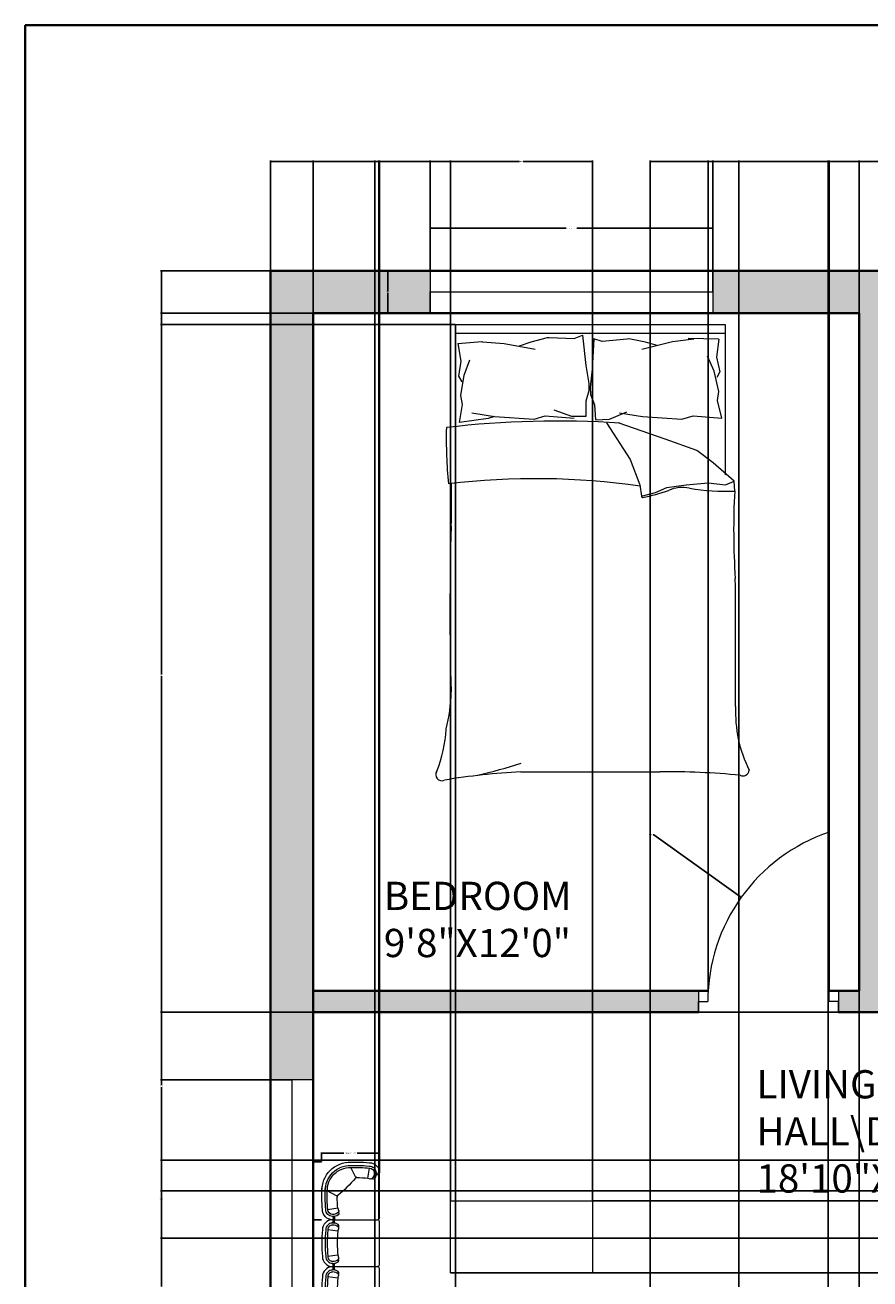
# Model space of a CAD drawing. Units: inches. Extents: x 2606 to 3027, y 1906 to 2463.
# Tile 5 of 10: x 2606 to 2785, y 2196 to 2463. Entities that reach past the tile are written whole.
import ezdxf

# ---------------------------------------------------------------- set-up
doc = ezdxf.new("R2010")
doc.units = ezdxf.units.IN
for name, color, linetype, lineweight in [('A-ANNO-DIMS', 2, 'Continuous', 18), ('A-ANNO-TTLB', 7, 'Continuous', 35), ('A-AREA-IDEN', 7, 'Continuous', 18), ('A-DOOR', 3, 'Continuous', 18), ('A-FURN', 8, 'Continuous', 13), ('A-GLAZ', 4, 'Continuous', 18), ('A-WALL', 7, 'Continuous', 35)]:
    doc.layers.add(name, color=color, linetype=linetype, lineweight=lineweight)
doc.layers.add('A-WALL-PATT', color=251, linetype='Continuous', lineweight=13, true_color=0x636466)
doc.styles.get("Standard").update_dxf_attribs({"font": 'arial.ttf'})
doc.dimstyles.get("Standard").update_dxf_attribs({"dimtxt": 0.18, "dimasz": 0.18, "dimexe": 0.18, "dimexo": 0.0625, "dimgap": 0.09, "dimtad": 0, "dimtih": 1, "dimtoh": 1, "dimdec": 4, "dimzin": 0, "dimdsep": 46, "dimtxsty": 'Standard', "dimcen": 0.09, "dimadec": 0, "dimazin": 0, "dimtfac": 1, "dimtdec": 4, "dimtofl": 0, "dimtmove": 0, "dimatfit": 3, "dimfxl": 1, "dimtolj": 1, "dimtzin": 0, "dimarcsym": 0})

# ---------------------------------------------------------------- blocks, each defined once
blk = doc.blocks.new('part 01')
at = {"color": 0}
for p, q in [((-670, 700), (0, 700)), ((-591, 527), (-579, 561)), ((30, 30), (30, 670)), ((-591, 527), (-740, 550)), ((-591, 173), (-740, 150)), ((-670, 0), (0, 0)), ((-591, 173), (-579, 139))]:
    blk.add_line(p, q, dxfattribs=at)
for centre, radius, start, end in [((-670, 550), 150, 90, 181.1754), ((-670, 550), 100, 90, 181.1754), ((-670, 550), 70, 90, 181.1754), ((-660, 518), 133, 56.0897, 95.6132), ((-696, 675), 36.2, 316.3972, 43.6028), ((-660, 518), 103, 42.0066, 95.6132), ((-706, 675), 66.2, 337.8298, 22.1702), ((-600, 607), 25, 332.9608, 56.0897), ((-625, 620), 53.2, 321.0017, 332.9608), ((-602, 570), 25, 340, 42.0066), ((0, 670), 30, 0, 90), ((1178, 350), 2008, 174.2835, 185.7165), ((1178, 350), 1958, 174.2835, 185.7165), ((1178, 350), 1928, 174.2835, 185.7165), ((1178, 350), 1778, 174.2835, 185.7165), ((-670, 150), 150, 178.8246, 270), ((-670, 150), 100, 178.8246, 270), ((-670, 150), 70, 178.8246, 270), ((-660, 182), 133, 264.3868, 303.9103), ((-660, 182), 103, 264.3868, 317.9934), ((-696, 25), 36.2, 316.3972, 43.6028), ((-706, 25), 66.2, 337.8298, 22.1702), ((-600, 93), 25, 303.9103, 27.0392), ((-602, 130), 25, 317.9934, 20), ((-625, 80), 53.2, 27.0392, 38.9983), ((0, 30), 30, 270, 0)]:
    blk.add_arc(centre, radius, start, end, dxfattribs=at)
blk = doc.blocks.new('part02')
at = {"color": 0}
for p, q in [((0, -670), (0, 0)), ((30, 30), (700, 30)), ((621, -143), (609, -109)), ((621, -143), (770, -120)), ((640, -326), (778, -399)), ((173, -591), (139, -579)), ((173, -591), (150, -740)), ((356, -610), (429, -748))]:
    blk.add_line(p, q, dxfattribs=at)
for centre, radius, start, end in [((30, 0), 30, 90, 180), ((726, 5), 56.2, 153.6122, 206.6666), ((726, 5), 36.2, 136.3972, 223.6028), ((700, -120), 150, 0, 90), ((630, -63), 25, 123.9103, 207.0392), ((655, -50), 53.2, 207.0392, 218.9983), ((632, -100), 25, 137.9934, 200), ((690, -152), 103, 84.3868, 137.9934), ((689, -151), 132, 85.4378, 123.9887), ((-1148, -320), 1778, 0.3836, 5.7165), ((700, -121), 101, 357.5006, 89.858), ((700, -120), 70, 0, 90), ((-1228, -320), 2008, 357.7349, 5.7032), ((-1148, -320), 1958, 355.8657, 5.7165), ((-1148, -320), 2008, 355.818, 5.7165), ((2220, -2190), 2454, 130.6961, 139.3039), ((632, -344), 20, 62, 130.6961), ((650, -308), 20, 180.3836, 242), ((439, -409), 419, 268.2181, 1.7819), ((439, -409), 369, 268.2181, 1.7819), ((439, -409), 339, 268.2181, 1.7819), ((25, -696), 56.2, 63.3334, 116.3878), ((25, -696), 36.2, 46.3972, 133.6028), ((150, -670), 150, 180, 271.1754), ((182, -660), 133, 146.0897, 185.6132), ((150, -670), 100, 180, 271.1754), ((93, -600), 25, 62.9608, 146.0897), ((182, -660), 103, 132.0066, 185.6132), ((150, -670), 70, 180, 270), ((80, -625), 53.2, 51.0017, 62.9608), ((130, -602), 25, 70, 132.0066), ((350, 1258), 2008, 264.2968, 272.2651), ((350, 1178), 1778, 264.2835, 269.6164), ((338, -620), 20, 28, 89.6164), ((374, -602), 20, 139.3039, 208), ((350, 1178), 2008, 264.2835, 274.182), ((350, 1178), 1958, 264.2835, 274.1343)]:
    blk.add_arc(centre, radius, start, end, dxfattribs=at)
blk = doc.blocks.new('BED-DOUBLE')
for p, q in [((4.17, 75.16), (4.17, 96.87)), ((4.17, 96.87), (61.46, 96.87)), ((61.46, 96.87), (61.46, 64.97)), ((4.17, 95.03), (61.46, 95.03)), ((4.67, 92.87), (9.81, 93.27)), ((9.81, 93.27), (9.93, 93.24)), ((9.93, 93.24), (14.52, 92.9)), ((17.81, 92.38), (20.24, 93.24)), ((20.24, 93.24), (23.7, 94.11)), ((23.7, 94.11), (24.09, 94.11)), ((24.09, 94.11), (29.42, 93.94)), ((29.42, 93.94), (31.15, 94.63)), ((31.15, 94.63), (31.84, 88.22)), ((33.54, 93.89), (33.25, 87.44)), ((35.31, 93.3), (33.54, 93.89)), ((40.62, 93.81), (35.31, 93.3)), ((41.01, 93.83), (40.62, 93.81)), ((44.52, 93.18), (41.01, 93.83)), ((54.8, 93.82), (50.25, 93.19)), ((60.08, 93.81), (53.6, 93.92)), ((53.6, 93.92), (54.8, 93.82)), ((60.08, 93.81), (59.62, 89.96)), ((4.67, 92.9), (5.36, 89.08)), ((14.52, 92.9), (21.1, 91.68)), ((50.25, 93.19), (43.75, 91.57)), ((47, 92.47), (44.52, 93.18)), ((5.36, 89.08), (4.84, 85.96)), ((6.06, 86.14), (7.27, 89.43)), ((31.84, 88.22), (32.54, 84.4)), ((59.12, 86.97), (57.7, 90.18)), ((59.62, 89.96), (60.34, 86.88)), ((4.84, 85.96), (5.54, 84.75)), ((5.36, 81.8), (6.06, 86.14)), ((33.25, 87.44), (32.79, 83.59)), ((60.08, 82.69), (59.12, 86.97)), ((60.34, 86.88), (59.72, 85.62)), ((32.54, 82.84), (31.84, 80.59)), ((32.54, 84.4), (32.54, 82.84)), ((32.79, 83.59), (32.89, 82.03)), ((59.85, 80.77), (60.08, 82.69)), ((5.71, 79.9), (5.36, 81.8)), ((31.84, 80.59), (31.84, 77.38)), ((32.89, 82.03), (33.72, 79.83)), ((60.78, 77), (59.85, 80.77)), ((5.02, 76.08), (5.71, 79.9)), ((7.65, 78.14), (12.48, 77.34)), ((12.48, 77.34), (11.13, 76.95)), ((12.48, 77.34), (20.89, 76.82)), ((20.89, 76.82), (23.24, 77.49)), ((23.24, 77.49), (29.39, 77)), ((28.9, 77.38), (25.13, 78.68)), ((31.84, 77.38), (28.9, 77.38)), ((33.72, 79.83), (33.92, 76.62)), ((36.87, 76.8), (40.55, 78.34)), ((39.04, 78.14), (43.87, 77.34)), ((43.87, 77.34), (52.28, 76.82)), ((52.28, 76.82), (54.63, 77.49)), ((54.63, 77.49), (60.78, 77)), ((11.13, 76.95), (5.02, 76.08)), ((33.92, 76.62), (36.87, 76.8)), ((36.28, 76.03), (41.3, 68.25)), ((48.73, 72.52), (38.73, 76.03)), ((55.41, 70.1), (48.73, 72.52)), ((58.94, 67.51), (55.41, 70.1)), ((41.3, 68.25), (43.34, 62.87)), ((63.38, 63.61), (58.94, 67.51)), ((43.34, 62.87), (43.71, 60.45)), ((46.68, 61.2), (49.1, 62.31)), ((49.1, 62.31), (53.18, 62.87)), ((53.18, 62.87), (57.82, 63.24)), ((57.82, 63.24), (61.54, 62.87)), ((61.54, 62.87), (63.38, 63.61)), ((63.48, 61.52), (63.38, 63.61, 4.64)), ((43.71, 60.45), (46.68, 61.2)), ((18.06, 1.87), (47.57, 1.87))]:
    blk.add_line(p, q)
for centre, radius, start, end in [((102.1, 72.78), 99.87, 178.7218, 185.604), ((25.61, -121.38), 197.77, 86.0865, 96.7821), ((21.29, -90.53), 154.68, 81.7845, 96.9006), ((-200.58, 59.5), 203.94, 358.4762, 1.0082), ((37.35, 95.1), 35.55, 280.6617, 289.8806), ((52.44, 54.83), 7.46, 78.6608, 113.7384), ((61.53, 104.85), 43.38, 259.8763, 272.5657), ((218.51, 53.34), 155.25, 176.9791, 183.8365), ((43.92, 60.38), 0.221, 160.2464, 271.1377), ((581.23, 36.19), 578.22, 178.22771, 181.71854), ((-5405.34, 15.56), 5469.02, 0.00217, 0.28689), ((-32.25, 19.53), 35.53, 346.0648, 358.9113), ((91.3, 14.55), 27.65, 177.4714, 206.4681), ((-25.97, 12.62), 28.25, 337.9751, 356.652), ((-20.65, 125.3), 127.63, 283.3832, 287.7053), ((1.3, 1.3), 1.31, 146.1736, 293.4781), ((25.69, -143.9), 145.97, 92.9958, 99.4091), ((49.34, -157.62), 159.5, 84.4998, 90.6351), ((65.23, 2.32), 1.32, 242.6588, 356.02)]:
    blk.add_arc(centre, radius, start, end)
blk = doc.blocks.new('WIN-60IN')
for p, q in [((0, 9), (0, 0)), ((60, 4.5), (60, 9)), ((60, 9), (60, 0)), ((0, 0), (0, 4.5)), ((0, 4.5), (60, 4.5))]:
    blk.add_line(p, q)
blk = doc.blocks.new('*D11')
at = {"layer": 'A-ANNO-DIMS', "color": 0, "lineweight": -2, "transparency": 16777216}
for p, q in [((2691.97, 2410.67), (2691.97, 2419.79)), ((2692.15, 2419.61), (2720.85, 2419.61)), ((2751.79, 2419.61), (2723.09, 2419.61)), ((2751.97, 2410.67), (2751.97, 2419.79))]:
    blk.add_line(p, q, dxfattribs=at)
at = {"layer": 'A-ANNO-DIMS', "color": 0, "transparency": 16777216}
for points in [[(2692.15, 2419.64), (2692.15, 2419.58), (2691.97, 2419.61)], [(2751.79, 2419.64), (2751.79, 2419.58), (2751.97, 2419.61)]]:
    blk.add_solid(points, dxfattribs=at)
at = {"layer": 'Defpoints', "color": 0, "transparency": 16777216}
for p in [(2751.97, 2419.61), (2691.97, 2410.61), (2751.97, 2410.61)]:
    blk.add_point(p, dxfattribs=at)
at = {"layer": 'A-ANNO-DIMS', "color": 0, "transparency": 16777216, "insert": (2721.97, 2419.61), "char_height": 0.18, "attachment_point": 5}
blk.add_mtext('\\A1;WINDOW 60 TYP.', dxfattribs=at)
blk = doc.blocks.new('*D12')
at = {"layer": 'A-ANNO-DIMS', "color": 0, "lineweight": -2, "transparency": 16777216}
for p, q in [((2691.91, 2410.61), (2682.79, 2410.61)), ((2682.97, 2410.43), (2682.97, 2406.29)), ((2682.97, 2401.79), (2682.97, 2405.93)), ((2691.91, 2401.61), (2682.79, 2401.61))]:
    blk.add_line(p, q, dxfattribs=at)
at = {"layer": 'A-ANNO-DIMS', "color": 0, "transparency": 16777216}
for points in [[(2682.94, 2410.43), (2683, 2410.43), (2682.97, 2410.61)], [(2682.94, 2401.79), (2683, 2401.79), (2682.97, 2401.61)]]:
    blk.add_solid(points, dxfattribs=at)
at = {"layer": 'Defpoints', "color": 0, "transparency": 16777216}
for p in [(2682.97, 2410.61), (2691.97, 2410.61), (2691.97, 2401.61)]:
    blk.add_point(p, dxfattribs=at)
at = {"layer": 'A-ANNO-DIMS', "color": 0, "transparency": 16777216, "insert": (2682.97, 2406.11), "char_height": 0.18, "attachment_point": 5}
blk.add_mtext('\\A1;9 TYP.', dxfattribs=at)
blk = doc.blocks.new('*D19')
at = {"layer": 'A-ANNO-DIMS', "color": 0, "lineweight": -2, "transparency": 16777216}
for p, q in [((2668.89, 2221.35), (2668.89, 2223.31)), ((2669.07, 2223.13), (2673.63, 2223.13)), ((2680.99, 2223.13), (2676.43, 2223.13)), ((2681.17, 2221.35), (2681.17, 2223.31))]:
    blk.add_line(p, q, dxfattribs=at)
at = {"layer": 'A-ANNO-DIMS', "color": 0, "transparency": 16777216}
for points in [[(2669.07, 2223.16), (2669.07, 2223.1), (2668.89, 2223.13)], [(2680.99, 2223.16), (2680.99, 2223.1), (2681.17, 2223.13)]]:
    blk.add_solid(points, dxfattribs=at)
at = {"layer": 'Defpoints', "color": 0, "transparency": 16777216}
for p in [(2681.17, 2223.13), (2668.89, 2221.29), (2681.17, 2221.29)]:
    blk.add_point(p, dxfattribs=at)
at = {"layer": 'A-ANNO-DIMS', "color": 0, "transparency": 16777216, "insert": (2675.03, 2223.13), "char_height": 0.18, "attachment_point": 5}
blk.add_mtext('\\A1;END MODULE 12 TYP.', dxfattribs=at)
blk = doc.blocks.new('*D20')
at = {"layer": 'A-ANNO-DIMS', "color": 0, "lineweight": -2, "transparency": 16777216}
for p, q in [((2668.83, 2221.29), (2666.86, 2221.29)), ((2667.04, 2221.11), (2667.04, 2215.33)), ((2667.04, 2209.19), (2667.04, 2214.97)), ((2668.83, 2209.01), (2666.86, 2209.01))]:
    blk.add_line(p, q, dxfattribs=at)
at = {"layer": 'A-ANNO-DIMS', "color": 0, "transparency": 16777216}
for points in [[(2667.01, 2221.11), (2667.07, 2221.11), (2667.04, 2221.29)], [(2667.01, 2209.19), (2667.07, 2209.19), (2667.04, 2209.01)]]:
    blk.add_solid(points, dxfattribs=at)
at = {"layer": 'Defpoints', "color": 0, "transparency": 16777216}
for p in [(2667.04, 2221.29), (2668.89, 2221.29), (2668.89, 2209.01)]:
    blk.add_point(p, dxfattribs=at)
at = {"layer": 'A-ANNO-DIMS', "color": 0, "transparency": 16777216, "insert": (2667.04, 2215.15), "char_height": 0.18, "attachment_point": 5}
blk.add_mtext('\\A1;12 TYP.', dxfattribs=at)
blk = doc.blocks.new('*D27')
at = {"layer": 'A-ANNO-DIMS', "color": 0, "lineweight": -2, "transparency": 16777216}
for p, q in [((2658.06, 2410.67), (2658.06, 2433.99)), ((2658.24, 2433.81), (2674.64, 2433.81)), ((2691.79, 2433.81), (2675.39, 2433.81)), ((2691.97, 2410.67), (2691.97, 2433.99))]:
    blk.add_line(p, q, dxfattribs=at)
at = {"layer": 'A-ANNO-DIMS', "color": 0, "transparency": 16777216}
for points in [[(2658.24, 2433.84), (2658.24, 2433.78), (2658.06, 2433.81)], [(2691.79, 2433.84), (2691.79, 2433.78), (2691.97, 2433.81)]]:
    blk.add_solid(points, dxfattribs=at)
at = {"layer": 'Defpoints', "color": 0, "transparency": 16777216}
for p in [(2691.97, 2433.81), (2658.06, 2410.61), (2691.97, 2410.61)]:
    blk.add_point(p, dxfattribs=at)
at = {"layer": 'A-ANNO-DIMS', "color": 0, "transparency": 16777216, "insert": (2675.02, 2433.81), "char_height": 0.18, "attachment_point": 5}
blk.add_mtext('\\A1;33.91', dxfattribs=at)
blk = doc.blocks.new('*D28')
at = {"layer": 'A-ANNO-DIMS', "color": 0, "lineweight": -2, "transparency": 16777216}
for p, q in [((2751.97, 2410.67), (2751.97, 2433.99)), ((2752.15, 2433.81), (2778.09, 2433.81)), ((2804.82, 2433.81), (2778.88, 2433.81)), ((2805, 2410.67), (2805, 2433.99))]:
    blk.add_line(p, q, dxfattribs=at)
at = {"layer": 'A-ANNO-DIMS', "color": 0, "transparency": 16777216}
for points in [[(2752.15, 2433.84), (2752.15, 2433.78), (2751.97, 2433.81)], [(2804.82, 2433.84), (2804.82, 2433.78), (2805, 2433.81)]]:
    blk.add_solid(points, dxfattribs=at)
at = {"layer": 'Defpoints', "color": 0, "transparency": 16777216}
for p in [(2805, 2433.81), (2751.97, 2410.61), (2805, 2410.61)]:
    blk.add_point(p, dxfattribs=at)
at = {"layer": 'A-ANNO-DIMS', "color": 0, "transparency": 16777216, "insert": (2778.48, 2433.81), "char_height": 0.18, "attachment_point": 5}
blk.add_mtext('\\A1;53.03', dxfattribs=at)
blk = doc.blocks.new('*D31')
at = {"layer": 'A-ANNO-DIMS', "color": 0, "lineweight": -2, "transparency": 16777216}
for p, q in [((2658, 2410.61), (2634.68, 2410.61)), ((2634.86, 2410.43), (2634.86, 2324.84)), ((2634.86, 2238.89), (2634.86, 2324.48)), ((2658, 2238.71), (2634.68, 2238.71))]:
    blk.add_line(p, q, dxfattribs=at)
at = {"layer": 'A-ANNO-DIMS', "color": 0, "transparency": 16777216}
for points in [[(2634.83, 2410.43), (2634.89, 2410.43), (2634.86, 2410.61)], [(2634.83, 2238.89), (2634.89, 2238.89), (2634.86, 2238.71)]]:
    blk.add_solid(points, dxfattribs=at)
at = {"layer": 'Defpoints', "color": 0, "transparency": 16777216}
for p in [(2634.86, 2410.61), (2658.06, 2410.61), (2658.06, 2238.71)]:
    blk.add_point(p, dxfattribs=at)
at = {"layer": 'A-ANNO-DIMS', "color": 0, "transparency": 16777216, "insert": (2634.86, 2324.66), "char_height": 0.18, "attachment_point": 5}
blk.add_mtext('\\A1;171.9', dxfattribs=at)
blk = doc.blocks.new('*D32')
at = {"layer": 'A-ANNO-DIMS', "color": 0, "lineweight": -2, "transparency": 16777216}
for p, q in [((2667.06, 2032.67), (2667.06, 2433.99)), ((2667.24, 2433.81), (2673.16, 2433.81)), ((2679.99, 2433.81), (2674.07, 2433.81)), ((2680.17, 2032.67), (2680.17, 2433.99))]:
    blk.add_line(p, q, dxfattribs=at)
at = {"layer": 'A-ANNO-DIMS', "color": 0, "transparency": 16777216}
for points in [[(2667.24, 2433.84), (2667.24, 2433.78), (2667.06, 2433.81)], [(2679.99, 2433.84), (2679.99, 2433.78), (2680.17, 2433.81)]]:
    blk.add_solid(points, dxfattribs=at)
at = {"layer": 'Defpoints', "color": 0, "transparency": 16777216}
for p in [(2680.17, 2433.81), (2667.06, 2032.61), (2680.17, 2032.61)]:
    blk.add_point(p, dxfattribs=at)
at = {"layer": 'A-ANNO-DIMS', "color": 0, "transparency": 16777216, "insert": (2673.61, 2433.81), "char_height": 0.18, "attachment_point": 5}
blk.add_mtext('\\A1;13.102', dxfattribs=at)
blk = doc.blocks.new('*D38')
at = {"layer": 'A-ANNO-DIMS', "color": 0, "lineweight": -2, "transparency": 16777216}
for p, q in [((2783.06, 1993.17), (2783.06, 2433.99)), ((2783.24, 2433.81), (2785.05, 2433.81)), ((2787.38, 2433.81), (2785.57, 2433.81)), ((2787.56, 1993.17), (2787.56, 2433.99))]:
    blk.add_line(p, q, dxfattribs=at)
at = {"layer": 'A-ANNO-DIMS', "color": 0, "transparency": 16777216}
for points in [[(2783.24, 2433.84), (2783.24, 2433.78), (2783.06, 2433.81)], [(2787.38, 2433.84), (2787.38, 2433.78), (2787.56, 2433.81)]]:
    blk.add_solid(points, dxfattribs=at)
at = {"layer": 'Defpoints', "color": 0, "transparency": 16777216}
for p in [(2787.56, 2433.81), (2783.06, 1993.11), (2787.56, 1993.11)]:
    blk.add_point(p, dxfattribs=at)
at = {"layer": 'A-ANNO-DIMS', "color": 0, "transparency": 16777216, "insert": (2785.31, 2433.81), "char_height": 0.18, "attachment_point": 5}
blk.add_mtext('\\A1;4.5', dxfattribs=at)
blk = doc.blocks.new('*D42')
at = {"layer": 'A-ANNO-DIMS', "color": 0, "lineweight": -2, "transparency": 16777216}
for p, q in [((2750.95, 2257.67), (2750.95, 2433.99)), ((2751.13, 2433.81), (2763.42, 2433.81)), ((2776.49, 2433.81), (2764.21, 2433.81)), ((2776.67, 2257.67), (2776.67, 2433.99))]:
    blk.add_line(p, q, dxfattribs=at)
at = {"layer": 'A-ANNO-DIMS', "color": 0, "transparency": 16777216}
for points in [[(2751.13, 2433.84), (2751.13, 2433.78), (2750.95, 2433.81)], [(2776.49, 2433.84), (2776.49, 2433.78), (2776.67, 2433.81)]]:
    blk.add_solid(points, dxfattribs=at)
at = {"layer": 'Defpoints', "color": 0, "transparency": 16777216}
for p in [(2776.67, 2433.81), (2750.95, 2257.61), (2776.67, 2257.61)]:
    blk.add_point(p, dxfattribs=at)
at = {"layer": 'A-ANNO-DIMS', "color": 0, "transparency": 16777216, "insert": (2763.81, 2433.81), "char_height": 0.18, "attachment_point": 5}
blk.add_mtext('\\A1;25.72', dxfattribs=at)
blk = doc.blocks.new('*D47')
at = {"layer": 'A-ANNO-DIMS', "color": 0, "lineweight": -2, "transparency": 16777216}
for p, q in [((2757.51, 2028.17), (2757.51, 2433.99)), ((2757.69, 2433.81), (2766.59, 2433.81)), ((2776.27, 2433.81), (2767.36, 2433.81)), ((2776.45, 2028.17), (2776.45, 2433.99))]:
    blk.add_line(p, q, dxfattribs=at)
at = {"layer": 'A-ANNO-DIMS', "color": 0, "transparency": 16777216}
for points in [[(2757.69, 2433.84), (2757.69, 2433.78), (2757.51, 2433.81)], [(2776.27, 2433.84), (2776.27, 2433.78), (2776.45, 2433.81)]]:
    blk.add_solid(points, dxfattribs=at)
at = {"layer": 'Defpoints', "color": 0, "transparency": 16777216}
for p in [(2776.45, 2433.81), (2757.51, 2028.11), (2776.45, 2028.11)]:
    blk.add_point(p, dxfattribs=at)
at = {"layer": 'A-ANNO-DIMS', "color": 0, "transparency": 16777216, "insert": (2766.98, 2433.81), "char_height": 0.18, "attachment_point": 5}
blk.add_mtext('\\A1;18.94', dxfattribs=at)
blk = doc.blocks.new('*D50')
at = {"layer": 'A-ANNO-DIMS', "color": 0, "lineweight": -2, "transparency": 16777216}
for p, q in [((2776.67, 2257.67), (2776.67, 2433.99)), ((2776.85, 2433.81), (2779.47, 2433.81)), ((2782.88, 2433.81), (2780.26, 2433.81)), ((2783.06, 2257.67), (2783.06, 2433.99))]:
    blk.add_line(p, q, dxfattribs=at)
at = {"layer": 'A-ANNO-DIMS', "color": 0, "transparency": 16777216}
for points in [[(2776.85, 2433.84), (2776.85, 2433.78), (2776.67, 2433.81)], [(2782.88, 2433.84), (2782.88, 2433.78), (2783.06, 2433.81)]]:
    blk.add_solid(points, dxfattribs=at)
at = {"layer": 'Defpoints', "color": 0, "transparency": 16777216}
for p in [(2783.06, 2433.81), (2776.67, 2257.61), (2783.06, 2257.61)]:
    blk.add_point(p, dxfattribs=at)
at = {"layer": 'A-ANNO-DIMS', "color": 0, "transparency": 16777216, "insert": (2779.87, 2433.81), "char_height": 0.18, "attachment_point": 5}
blk.add_mtext('\\A1;6.389', dxfattribs=at)
blk = doc.blocks.new('*D56')
at = {"layer": 'A-ANNO-DIMS', "color": 0, "lineweight": -2, "transparency": 16777216}
for p, q in [((2776.45, 2028.17), (2776.45, 2433.99)), ((2776.63, 2433.81), (2779.36, 2433.81)), ((2782.88, 2433.81), (2780.15, 2433.81)), ((2783.06, 2032.67), (2783.06, 2433.99))]:
    blk.add_line(p, q, dxfattribs=at)
at = {"layer": 'A-ANNO-DIMS', "color": 0, "transparency": 16777216}
for points in [[(2776.63, 2433.84), (2776.63, 2433.78), (2776.45, 2433.81)], [(2782.88, 2433.84), (2782.88, 2433.78), (2783.06, 2433.81)]]:
    blk.add_solid(points, dxfattribs=at)
at = {"layer": 'Defpoints', "color": 0, "transparency": 16777216}
for p in [(2783.06, 2433.81), (2783.06, 2032.61), (2776.45, 2028.11)]:
    blk.add_point(p, dxfattribs=at)
at = {"layer": 'A-ANNO-DIMS', "color": 0, "transparency": 16777216, "insert": (2779.76, 2433.81), "char_height": 0.18, "attachment_point": 5}
blk.add_mtext('\\A1;6.615', dxfattribs=at)
blk = doc.blocks.new('*D58')
at = {"layer": 'A-ANNO-DIMS', "color": 0, "lineweight": -2, "transparency": 16777216}
for p, q in [((2696.23, 2213.1), (2696.23, 2433.99)), ((2696.41, 2433.81), (2710.92, 2433.81)), ((2726.22, 2433.81), (2711.71, 2433.81)), ((2726.4, 2213.1), (2726.4, 2433.99))]:
    blk.add_line(p, q, dxfattribs=at)
at = {"layer": 'A-ANNO-DIMS', "color": 0, "transparency": 16777216}
for points in [[(2696.41, 2433.84), (2696.41, 2433.78), (2696.23, 2433.81)], [(2726.22, 2433.84), (2726.22, 2433.78), (2726.4, 2433.81)]]:
    blk.add_solid(points, dxfattribs=at)
at = {"layer": 'Defpoints', "color": 0, "transparency": 16777216}
for p in [(2726.4, 2433.81), (2696.23, 2213.03), (2726.4, 2213.03)]:
    blk.add_point(p, dxfattribs=at)
at = {"layer": 'A-ANNO-DIMS', "color": 0, "transparency": 16777216, "insert": (2711.32, 2433.81), "char_height": 0.18, "attachment_point": 5}
blk.add_mtext('\\A1;30.17', dxfattribs=at)
blk = doc.blocks.new('*D59')
at = {"layer": 'A-ANNO-DIMS', "color": 0, "lineweight": -2, "transparency": 16777216}
for p, q in [((2726.47, 2213.03), (3000.44, 2213.03)), ((3000.26, 2212.85), (3000.26, 2205.56)), ((3000.26, 2197.9), (3000.26, 2205.2)), ((2726.47, 2197.72), (3000.44, 2197.72))]:
    blk.add_line(p, q, dxfattribs=at)
at = {"layer": 'A-ANNO-DIMS', "color": 0, "transparency": 16777216}
for points in [[(3000.23, 2212.85), (3000.29, 2212.85), (3000.26, 2213.03)], [(3000.23, 2197.9), (3000.29, 2197.9), (3000.26, 2197.72)]]:
    blk.add_solid(points, dxfattribs=at)
at = {"layer": 'Defpoints', "color": 0, "transparency": 16777216}
for p in [(2726.4, 2213.03), (3000.26, 2213.03), (2726.4, 2197.72)]:
    blk.add_point(p, dxfattribs=at)
at = {"layer": 'A-ANNO-DIMS', "color": 0, "transparency": 16777216, "insert": (3000.26, 2205.38), "char_height": 0.18, "attachment_point": 5}
blk.add_mtext('\\A1;15.31', dxfattribs=at)
blk = doc.blocks.new('*D60')
at = {"layer": 'A-ANNO-DIMS', "color": 0, "lineweight": -2, "transparency": 16777216}
for p, q in [((2681.05, 2209.19), (2681.05, 2433.99)), ((2681.23, 2433.81), (2688.19, 2433.81)), ((2696.05, 2433.81), (2689.1, 2433.81)), ((2696.23, 2213.1), (2696.23, 2433.99))]:
    blk.add_line(p, q, dxfattribs=at)
at = {"layer": 'A-ANNO-DIMS', "color": 0, "transparency": 16777216}
for points in [[(2681.23, 2433.84), (2681.23, 2433.78), (2681.05, 2433.81)], [(2696.05, 2433.84), (2696.05, 2433.78), (2696.23, 2433.81)]]:
    blk.add_solid(points, dxfattribs=at)
at = {"layer": 'Defpoints', "color": 0, "transparency": 16777216}
for p in [(2696.23, 2433.81), (2696.23, 2213.03), (2681.05, 2209.13)]:
    blk.add_point(p, dxfattribs=at)
at = {"layer": 'A-ANNO-DIMS', "color": 0, "transparency": 16777216, "insert": (2688.64, 2433.81), "char_height": 0.18, "attachment_point": 5}
blk.add_mtext('\\A1;15.184', dxfattribs=at)
blk = doc.blocks.new('*D61')
at = {"layer": 'A-ANNO-DIMS', "color": 0, "lineweight": -2, "transparency": 16777216}
for p, q in [((2696.29, 2197.72), (3000.44, 2197.72)), ((3000.26, 2197.54), (3000.26, 2190.63)), ((3000.26, 2183.36), (3000.26, 2190.27)), ((2696.84, 2183.18), (3000.44, 2183.18))]:
    blk.add_line(p, q, dxfattribs=at)
at = {"layer": 'A-ANNO-DIMS', "color": 0, "transparency": 16777216}
for points in [[(3000.23, 2197.54), (3000.29, 2197.54), (3000.26, 2197.72)], [(3000.23, 2183.36), (3000.29, 2183.36), (3000.26, 2183.18)]]:
    blk.add_solid(points, dxfattribs=at)
at = {"layer": 'Defpoints', "color": 0, "transparency": 16777216}
for p in [(2696.23, 2197.72), (3000.26, 2197.72), (2696.78, 2183.18)]:
    blk.add_point(p, dxfattribs=at)
at = {"layer": 'A-ANNO-DIMS', "color": 0, "transparency": 16777216, "insert": (3000.26, 2190.45), "char_height": 0.18, "attachment_point": 5}
blk.add_mtext('\\A1;14.545', dxfattribs=at)
blk = doc.blocks.new('*D63')
at = {"layer": 'A-ANNO-DIMS', "color": 0, "lineweight": -2, "transparency": 16777216}
for p, q in [((2667.06, 2238.77), (2667.06, 2433.99)), ((2667.24, 2433.81), (2673.75, 2433.81)), ((2680.99, 2433.81), (2674.49, 2433.81)), ((2681.17, 2219.03), (2681.17, 2433.99))]:
    blk.add_line(p, q, dxfattribs=at)
at = {"layer": 'A-ANNO-DIMS', "color": 0, "transparency": 16777216}
for points in [[(2667.24, 2433.84), (2667.24, 2433.78), (2667.06, 2433.81)], [(2680.99, 2433.84), (2680.99, 2433.78), (2681.17, 2433.81)]]:
    blk.add_solid(points, dxfattribs=at)
at = {"layer": 'Defpoints', "color": 0, "transparency": 16777216}
for p in [(2681.17, 2433.81), (2667.06, 2238.71), (2681.17, 2218.97)]:
    blk.add_point(p, dxfattribs=at)
at = {"layer": 'A-ANNO-DIMS', "color": 0, "transparency": 16777216, "insert": (2674.12, 2433.81), "char_height": 0.18, "attachment_point": 5}
blk.add_mtext('\\A1;14.11', dxfattribs=at)
blk = doc.blocks.new('*D68')
at = {"layer": 'A-ANNO-DIMS', "color": 0, "lineweight": -2, "transparency": 16777216}
for p, q in [((2897, 2215.13), (2634.68, 2215.13)), ((2634.86, 2214.95), (2634.86, 2194.85)), ((2634.86, 2174.38), (2634.86, 2194.48)), ((2897, 2174.2), (2634.68, 2174.2))]:
    blk.add_line(p, q, dxfattribs=at)
at = {"layer": 'A-ANNO-DIMS', "color": 0, "transparency": 16777216}
for points in [[(2634.83, 2214.95), (2634.89, 2214.95), (2634.86, 2215.13)], [(2634.83, 2174.38), (2634.89, 2174.38), (2634.86, 2174.2)]]:
    blk.add_solid(points, dxfattribs=at)
at = {"layer": 'Defpoints', "color": 0, "transparency": 16777216}
for p in [(2897.06, 2215.13), (2634.86, 2174.2), (2897.06, 2174.2)]:
    blk.add_point(p, dxfattribs=at)
at = {"layer": 'A-ANNO-DIMS', "color": 0, "transparency": 16777216, "insert": (2634.86, 2194.66), "char_height": 0.18, "attachment_point": 5}
blk.add_mtext('\\A1;40.94', dxfattribs=at)
blk = doc.blocks.new('*D71')
at = {"layer": 'A-ANNO-DIMS', "color": 0, "lineweight": -2, "transparency": 16777216}
for p, q in [((2847.16, 2221.64), (2634.68, 2221.64)), ((2634.86, 2221.46), (2634.86, 2213.56)), ((2634.86, 2205.29), (2634.86, 2213.19)), ((2847.16, 2205.11), (2634.68, 2205.11))]:
    blk.add_line(p, q, dxfattribs=at)
at = {"layer": 'A-ANNO-DIMS', "color": 0, "transparency": 16777216}
for points in [[(2634.83, 2221.46), (2634.89, 2221.46), (2634.86, 2221.64)], [(2634.83, 2205.29), (2634.89, 2205.29), (2634.86, 2205.11)]]:
    blk.add_solid(points, dxfattribs=at)
at = {"layer": 'Defpoints', "color": 0, "transparency": 16777216}
for p in [(2847.23, 2221.64), (2634.86, 2205.11), (2847.23, 2205.11)]:
    blk.add_point(p, dxfattribs=at)
at = {"layer": 'A-ANNO-DIMS', "color": 0, "transparency": 16777216, "insert": (2634.86, 2213.37), "char_height": 0.18, "attachment_point": 5}
blk.add_mtext('\\A1;16.533', dxfattribs=at)
blk = doc.blocks.new('*D73')
at = {"layer": 'A-ANNO-DIMS', "color": 0, "lineweight": -2, "transparency": 16777216}
for p, q in [((2886.91, 2253.11), (2634.68, 2253.11)), ((2634.86, 2252.93), (2634.86, 2237.56)), ((2634.86, 2221.82), (2634.86, 2237.19)), ((2847.16, 2221.64), (2634.68, 2221.64))]:
    blk.add_line(p, q, dxfattribs=at)
at = {"layer": 'A-ANNO-DIMS', "color": 0, "transparency": 16777216}
for points in [[(2634.83, 2252.93), (2634.89, 2252.93), (2634.86, 2253.11)], [(2634.83, 2221.82), (2634.89, 2221.82), (2634.86, 2221.64)]]:
    blk.add_solid(points, dxfattribs=at)
at = {"layer": 'Defpoints', "color": 0, "transparency": 16777216}
for p in [(2634.86, 2253.11), (2886.97, 2253.11), (2847.23, 2221.64)]:
    blk.add_point(p, dxfattribs=at)
at = {"layer": 'A-ANNO-DIMS', "color": 0, "transparency": 16777216, "insert": (2634.86, 2237.37), "char_height": 0.18, "attachment_point": 5}
blk.add_mtext('\\A1;31.47', dxfattribs=at)
blk = doc.blocks.new('*D74')
at = {"layer": 'A-ANNO-DIMS', "color": 0, "lineweight": -2, "transparency": 16777216}
for p, q in [((2667.06, 2401.55), (2667.06, 1965.23)), ((2697.29, 2399.09), (2697.29, 1965.23)), ((2667.24, 1965.41), (2681.71, 1965.41)), ((2697.11, 1965.41), (2682.64, 1965.41))]:
    blk.add_line(p, q, dxfattribs=at)
at = {"layer": 'A-ANNO-DIMS', "color": 0, "transparency": 16777216}
for points in [[(2667.24, 1965.44), (2667.24, 1965.38), (2667.06, 1965.41)], [(2697.11, 1965.44), (2697.11, 1965.38), (2697.29, 1965.41)]]:
    blk.add_solid(points, dxfattribs=at)
at = {"layer": 'Defpoints', "color": 0, "transparency": 16777216}
for p in [(2667.06, 2401.61), (2697.29, 2399.15), (2667.06, 1965.41)]:
    blk.add_point(p, dxfattribs=at)
at = {"layer": 'A-ANNO-DIMS', "color": 0, "transparency": 16777216, "insert": (2682.18, 1965.41), "char_height": 0.18, "attachment_point": 5}
blk.add_mtext('\\A1;30.225', dxfattribs=at)
blk = doc.blocks.new('*D76')
at = {"layer": 'A-ANNO-DIMS', "color": 0, "lineweight": -2, "transparency": 16777216}
for p, q in [((2738.62, 2035.66), (2738.62, 2433.99)), ((2738.8, 2433.81), (2760.37, 2433.81)), ((2782.88, 2433.81), (2761.31, 2433.81)), ((2783.06, 2032.67), (2783.06, 2433.99))]:
    blk.add_line(p, q, dxfattribs=at)
at = {"layer": 'A-ANNO-DIMS', "color": 0, "transparency": 16777216}
for points in [[(2738.8, 2433.84), (2738.8, 2433.78), (2738.62, 2433.81)], [(2782.88, 2433.84), (2782.88, 2433.78), (2783.06, 2433.81)]]:
    blk.add_solid(points, dxfattribs=at)
at = {"layer": 'Defpoints', "color": 0, "transparency": 16777216}
for p in [(2783.06, 2433.81), (2738.62, 2035.6), (2783.06, 2032.61)]:
    blk.add_point(p, dxfattribs=at)
at = {"layer": 'A-ANNO-DIMS', "color": 0, "transparency": 16777216, "insert": (2760.84, 2433.81), "char_height": 0.18, "attachment_point": 5}
blk.add_mtext('\\A1;44.445', dxfattribs=at)
blk = doc.blocks.new('*D78')
at = {"layer": 'A-ANNO-DIMS', "color": 0, "lineweight": -2, "transparency": 16777216}
for p, q in [((2691.91, 2401.61), (2634.68, 2401.61)), ((2634.86, 2401.43), (2634.86, 2400.56)), ((2634.86, 2399.33), (2634.86, 2400.2)), ((2697.23, 2399.15), (2634.68, 2399.15))]:
    blk.add_line(p, q, dxfattribs=at)
at = {"layer": 'A-ANNO-DIMS', "color": 0, "transparency": 16777216}
for points in [[(2634.83, 2401.43), (2634.89, 2401.43), (2634.86, 2401.61)], [(2634.83, 2399.33), (2634.89, 2399.33), (2634.86, 2399.15)]]:
    blk.add_solid(points, dxfattribs=at)
at = {"layer": 'Defpoints', "color": 0, "transparency": 16777216}
for p in [(2634.86, 2401.61), (2691.97, 2401.61), (2697.29, 2399.15)]:
    blk.add_point(p, dxfattribs=at)
at = {"layer": 'A-ANNO-DIMS', "color": 0, "transparency": 16777216, "insert": (2634.86, 2400.38), "char_height": 0.18, "attachment_point": 5}
blk.add_mtext('\\A1;2.46', dxfattribs=at)
blk = doc.blocks.new('*D84')
at = {"layer": 'A-ANNO-DIMS', "color": 0, "lineweight": -2, "transparency": 16777216}
for p, q in [((2739.27, 2290.79), (2739.45, 2290.79)), ((2739.45, 2290.79), (2757.85, 2277.61)), ((2788.82, 2255.36), (2789, 2255.36)), ((2788.91, 2255.27), (2788.91, 2255.45))]:
    blk.add_line(p, q, dxfattribs=at)
at = {"layer": 'A-ANNO-DIMS', "color": 0, "transparency": 16777216}
blk.add_solid([(2757.87, 2277.63), (2757.84, 2277.58), (2758, 2277.5)], dxfattribs=at)
at = {"layer": 'Defpoints', "color": 0, "transparency": 16777216}
for p in [(2758, 2277.5), (2788.91, 2255.36)]:
    blk.add_point(p, dxfattribs=at)
at = {"layer": 'A-ANNO-DIMS', "color": 0, "transparency": 16777216, "insert": (2738.79, 2290.79), "char_height": 0.18, "attachment_point": 5}
blk.add_mtext('\\A1;R38.02', dxfattribs=at)

msp = doc.modelspace()

# ---------------------------------------------------------------- hatches: boundary and pattern name
at = {"layer": 'A-WALL-PATT'}
h = msp.add_hatch(color=256, dxfattribs=at)
h.dxf.hatch_style = 1
h.paths.add_polyline_path([(2667.063, 2401.6097), (2691.9697, 2401.6097), (2691.9697, 2406.1097), (2691.9697, 2410.6097), (2658.063, 2410.6097), (2658.063, 2238.7051), (2667.063, 2238.7051)])
h.paths.add_polyline_path([(2804.9965, 2406.1097), (2804.9965, 2410.6097), (2751.9697, 2410.6097), (2751.9697, 2401.6097), (2783.063, 2401.6097), (2783.063, 2257.6097), (2778.6739, 2257.6097), (2778.6739, 2253.1097), (2792.3386, 2253.1097), (2792.3386, 2255.3597), (2792.3386, 2257.6097), (2787.563, 2257.6097), (2787.563, 2327.1097), (2847.563, 2327.1097), (2847.563, 2331.6097), (2787.563, 2331.6097), (2787.563, 2401.6097), (2804.9965, 2401.6097)])
h.paths.add_polyline_path([(2889.6183, 2406.1097), (2889.6183, 2410.6097), (2828.9965, 2410.6097), (2828.9965, 2401.6097), (2831.8174, 2401.6097), (2847.563, 2401.6097), (2847.563, 2357.8311), (2849.813, 2357.8311), (2852.063, 2357.8311), (2852.063, 2401.6097), (2889.6183, 2401.6097)])
h.paths.add_polyline_path([(2977.063, 2410.6097), (2949.6183, 2410.6097), (2949.6183, 2401.6097), (2968.063, 2401.6097), (2968.063, 2157.1097), (2897.063, 2157.1097), (2897.063, 2174.1966), (2892.563, 2174.1966), (2892.563, 2157.1097), (2886.8122, 2157.1097), (2886.8122, 2152.6097), (2968.063, 2152.6097), (2968.063, 2032.6097), (2950.8911, 2032.6097), (2950.8911, 2028.1097), (2968.063, 2028.1097), (2968.063, 1993.1097), (2852.063, 1993.1097), (2852.063, 2028.1097), (2856.0743, 2028.1097), (2856.0743, 2030.3597), (2856.0743, 2032.6097), (2852.063, 2032.6097), (2852.063, 2152.6097), (2857.369, 2152.6097), (2857.369, 2154.8597), (2857.369, 2157.1097), (2847.563, 2157.1097), (2847.563, 2152.6097), (2847.563, 1993.1097), (2837.0415, 1993.1097), (2837.0415, 1988.6097), (2977.063, 1988.6097)])
h.paths.add_polyline_path([(2968.063, 2257.6097), (2886.9679, 2257.6097), (2886.9679, 2253.1097), (2892.563, 2253.1097), (2892.563, 2215.1332), (2897.063, 2215.1332), (2897.063, 2253.1097), (2968.063, 2253.1097)], flags=17)
h.paths.add_polyline_path([(2856.057, 2255.3597), (2856.057, 2257.6097), (2852.063, 2257.6097), (2852.063, 2336.7476), (2849.813, 2336.7476), (2847.563, 2336.7476), (2847.563, 2331.6097), (2847.563, 2327.1097), (2847.563, 2257.6097), (2813.482, 2257.6097), (2813.482, 2253.1097), (2856.057, 2253.1097)])
h.paths.add_polyline_path([(2748.8874, 2255.3597), (2748.8874, 2257.6097), (2667.063, 2257.6097), (2667.063, 2253.1097), (2748.8874, 2253.1097)])
h.paths.add_polyline_path([(2667.063, 2152.6097), (2744.8238, 2152.6097), (2744.8238, 2154.8597), (2744.8238, 2157.1097), (2667.063, 2157.1097), (2667.063, 2178.7051), (2658.063, 2178.7051), (2658.063, 1988.6097), (2801.0415, 1988.6097), (2801.0415, 1990.8597), (2801.0415, 1993.1097), (2787.563, 1993.1097), (2787.563, 2157.1097), (2777.1295, 2157.1097), (2777.1295, 2152.6097), (2783.063, 2152.6097), (2783.063, 2032.6097), (2778.4484, 2032.6097), (2778.4484, 2028.1097), (2783.063, 2028.1097), (2783.063, 1993.1097), (2667.063, 1993.1097), (2667.063, 2028.1097), (2680.1652, 2028.1097), (2680.1652, 2030.3597), (2680.1652, 2032.6097), (2667.063, 2032.6097)])
h.paths.add_polyline_path([(2755.4074, 2032.6097), (2728.1652, 2032.6097), (2728.1652, 2028.1097), (2755.4074, 2028.1097), (2755.4074, 2030.3597)], flags=17)
h.paths.add_polyline_path([(2902.8911, 2030.3597), (2902.8911, 2032.6097), (2877.6885, 2032.6097), (2877.6885, 2028.1097), (2902.8911, 2028.1097)], flags=17)
h.paths.add_polyline_path([(2810.2211, 2267.221), (2851.2716, 2267.221), (2851.2716, 2289.6098), (2810.2211, 2289.6098)], flags=9)

# ---------------------------------------------------------------- linework, layer by layer
at = {"layer": 'A-ANNO-TTLB'}
msp.add_lwpolyline([(2605.9227, 2462.7868), (3027.4339, 2462.7868), (3027.4339, 1905.5336), (2605.9227, 1905.5336)], close=True, dxfattribs=at)
at = {"layer": 'A-DOOR'}
for p, q in [((2776.6739, 2255.3597), (2776.6739, 2291.3597)), ((2748.8874, 2257.6097), (2748.8874, 2253.1097)), ((2778.6739, 2257.6097), (2778.6739, 2253.1097)), ((2748.8874, 2253.1097), (2748.8874, 2255.3597)), ((2748.8874, 2255.3597), (2750.8874, 2255.3597)), ((2778.6739, 2255.3597), (2776.6739, 2255.3597)), ((2778.6739, 2253.1097), (2778.6739, 2255.3597))]:
    msp.add_line(p, q, dxfattribs=at)
msp.add_arc((2788.9101, 2255.3597), 38.0227, 108.77262, 180, dxfattribs=at)
at = {"layer": 'A-FURN'}
msp.add_lwpolyline([(2696.232, 2213.0343), (2726.4032, 2213.0343), (2726.4032, 2197.7249), (2696.232, 2197.7249)], close=True, dxfattribs=at)
at = {"layer": 'A-WALL'}
for p, q in [((2658.063, 2410.6097), (2977.063, 2410.6097)), ((2658.063, 2410.6097), (2658.063, 1988.6097)), ((2667.063, 2401.6097), (2783.063, 2401.6097)), ((2667.063, 2401.6097), (2667.063, 2157.1097)), ((2783.063, 2401.6097), (2783.063, 2257.6097)), ((2667.063, 2257.6097), (2750.954, 2257.6097)), ((2776.6739, 2257.6097), (2783.063, 2257.6097)), ((2667.063, 2253.1097), (2748.8874, 2253.1097)), ((2778.6739, 2253.1097), (2792.3386, 2253.1097))]:
    msp.add_line(p, q, dxfattribs=at)

# ---------------------------------------------------------------- block references
at = {"layer": 'A-FURN'}
msp.add_blockref('BED-DOUBLE', (2693.1215, 2302.2788), dxfattribs=at)
at = {"layer": 'A-FURN', "ltscale": 0.03, "xscale": -0.0142384057136167, "yscale": 0.0142384057136167, "zscale": 0.0142384057136167, "rotation": 269.9999999999968}
msp.add_blockref('part02', (2680.7465, 2209.0056), dxfattribs=at)
at = {"layer": 'A-FURN', "ltscale": 0.03, "xscale": 0.0142384057136167, "yscale": 0.0142384057136167, "zscale": 0.0142384057136167}
for p in [(2680.7465, 2199.0387), (2680.7465, 2189.0719)]:
    msp.add_blockref('part 01', p, dxfattribs=at)
at = {"layer": 'A-GLAZ'}
msp.add_blockref('WIN-60IN', (2691.97, 2401.61), dxfattribs=at)
at = {"layer": 'A-GLAZ', "rotation": 270.0000000000001}
msp.add_blockref('WIN-60IN', (2658.0633, 2238.7048), dxfattribs=at)

# ---------------------------------------------------------------- texts
at = {"layer": 'A-AREA-IDEN', "char_height": 6, "attachment_point": 1}
for s, width, insert in [('BEDROOM\\P9\'8"X12\'0"', 64.066467, (2682.1187, 2280.7955)), ('LIVING HALL\\\\DINING \\P18\'10"X8\'0"', 67.964432, (2761.2312, 2240.7798))]:
    msp.add_mtext_dynamic_manual_height_columns(s, width=width, gutter_width=12.5, heights=[0], dxfattribs=dict(at, insert=insert))

# ---------------------------------------------------------------- dimensions: what is measured, and where the dimension line sits
at = {"layer": 'A-ANNO-DIMS'}
for base, p1, p2, override, picture, middle in [((2691.9697, 2433.8097), (2658.063, 2410.6097), (2691.9697, 2410.6097), {"dimdec": 2, "dimlfac": 1, "dimrnd": 0, "dimzin": 0, "dimdsep": 46, "dimlunit": 2}, '*D27', (2675.0163, 2433.8097)), ((2680.1652, 2433.8097), (2667.063, 2032.6097), (2680.1652, 2032.6097), {"dimdec": 3, "dimlfac": 1, "dimrnd": 0, "dimzin": 0, "dimdsep": 46, "dimlunit": 2}, '*D32', (2673.6141, 2433.8097)), ((2681.1736, 2433.8097), (2667.063, 2238.7051), (2681.1736, 2218.9696), {"dimdec": 2, "dimlfac": 1, "dimrnd": 0, "dimzin": 0, "dimdsep": 46, "dimlunit": 2}, '*D63', (2674.1183, 2433.8097)), ((2696.232034, 2433.809696), (2681.048527, 2209.130743), (2696.232034, 2213.03426), {"dimdec": 3, "dimlfac": 1, "dimrnd": 0, "dimzin": 0, "dimdsep": 46, "dimlunit": 2}, '*D60', (2688.64028, 2433.809696)), ((2726.4032, 2433.8097), (2696.232, 2213.0343), (2726.4032, 2213.0343), {"dimdec": 2, "dimlfac": 1, "dimrnd": 0, "dimzin": 0, "dimdsep": 46, "dimlunit": 2}, '*D58', (2711.3176, 2433.8097)), ((2783.063, 2433.8097), (2738.6178, 2035.5977), (2783.063, 2032.6097), {"dimdec": 3, "dimlfac": 1, "dimrnd": 0, "dimzin": 0, "dimdsep": 46, "dimlunit": 2}, '*D76', (2760.8404, 2433.8097)), ((2776.6739, 2433.8097), (2750.954, 2257.6097), (2776.6739, 2257.6097), {"dimdec": 2, "dimlfac": 1, "dimrnd": 0, "dimzin": 0, "dimdsep": 46, "dimlunit": 2}, '*D42', (2763.8139, 2433.8097)), ((2804.9965, 2433.8097), (2751.9697, 2410.6097), (2804.9965, 2410.6097), {"dimdec": 2, "dimlfac": 1, "dimrnd": 0, "dimzin": 0, "dimdsep": 46, "dimlunit": 2}, '*D28', (2778.4831, 2433.8097)), ((2776.4484, 2433.8097), (2757.5103, 2028.1097), (2776.4484, 2028.1097), {"dimdec": 2, "dimlfac": 1, "dimrnd": 0, "dimzin": 0, "dimdsep": 46, "dimlunit": 2}, '*D47', (2766.9794, 2433.8097)), ((2783.063, 2433.8097), (2776.4484, 2028.1097), (2783.063, 2032.6097), {"dimdec": 3, "dimlfac": 1, "dimrnd": 0, "dimzin": 0, "dimdsep": 46, "dimlunit": 2}, '*D56', (2779.7557, 2433.8097)), ((2783.063, 2433.8097), (2776.6739, 2257.6097), (2783.063, 2257.6097), {"dimdec": 3, "dimlfac": 1, "dimrnd": 0, "dimzin": 0, "dimdsep": 46, "dimlunit": 2}, '*D50', (2779.8684, 2433.8097)), ((2787.563, 2433.8097), (2783.063, 1993.1097), (2787.563, 1993.1097), {"dimdec": 1, "dimlfac": 1, "dimrnd": 0, "dimzin": 0, "dimdsep": 46, "dimlunit": 2}, '*D38', (2785.313, 2433.8097)), ((2667.063, 1965.4097), (2697.2878, 2399.1511), (2667.063, 2401.6097), {"dimdec": 3, "dimlfac": 1, "dimrnd": 0, "dimzin": 0, "dimdsep": 46, "dimlunit": 2}, '*D74', (2682.1754, 1965.4097))]:
    dim = msp.add_linear_dim(base=base, p1=p1, p2=p2, dimstyle='Standard', override=override, dxfattribs=at)
    dim.commit()
    dim.dimension.update_dxf_attribs({"geometry": picture, "text_midpoint": middle})
for base, p1, p2, text, picture, middle in [((2751.9697, 2419.6097), (2691.9697, 2410.6097), (2751.9697, 2410.6097), 'WINDOW <> TYP.', '*D11', (2721.9697, 2419.6097)), ((2681.1736, 2223.1344), (2668.8877, 2221.2915), (2681.1736, 2221.2915), 'END MODULE <> TYP.', '*D19', (2675.0307, 2223.1344))]:
    dim = msp.add_linear_dim(base=base, p1=p1, p2=p2, text=text, dimstyle='Standard', override={"dimdec": 0, "dimlfac": 1, "dimrnd": 0, "dimzin": 0, "dimdsep": 46, "dimlunit": 2}, dxfattribs=at)
    dim.commit()
    dim.dimension.update_dxf_attribs({"geometry": picture, "text_midpoint": middle})
for base, p1, p2, override, picture, middle in [((2634.863, 2410.6097), (2658.063, 2238.7051), (2658.063, 2410.6097), {"dimdec": 1, "dimlfac": 1, "dimrnd": 0, "dimzin": 0, "dimdsep": 46, "dimlunit": 2}, '*D31', (2634.863, 2324.6574)), ((2634.863, 2401.6097), (2697.2878, 2399.1511), (2691.9697, 2401.6097), {"dimdec": 2, "dimlfac": 1, "dimrnd": 0, "dimzin": 0, "dimdsep": 46, "dimlunit": 2}, '*D78', (2634.863, 2400.3804)), ((2634.863, 2253.1097), (2847.2251, 2221.6399), (2886.9679, 2253.1097), {"dimdec": 2, "dimlfac": 1, "dimrnd": 0, "dimzin": 0, "dimdsep": 46, "dimlunit": 2}, '*D73', (2634.863, 2237.3748)), ((2634.863, 2205.1069), (2847.2251, 2221.6399), (2847.2251, 2205.1069), {"dimdec": 3, "dimlfac": 1, "dimrnd": 0, "dimzin": 0, "dimdsep": 46, "dimlunit": 2}, '*D71', (2634.863, 2213.3734)), ((2634.863, 2174.1966), (2897.063, 2215.1332), (2897.063, 2174.1966), {"dimdec": 2, "dimlfac": 1, "dimrnd": 0, "dimzin": 0, "dimdsep": 46, "dimlunit": 2}, '*D68', (2634.863, 2194.6649)), ((3000.263, 2213.0343), (2726.4032, 2197.7249), (2726.4032, 2213.0343), {"dimdec": 2, "dimlfac": 1, "dimrnd": 0, "dimzin": 0, "dimdsep": 46, "dimlunit": 2}, '*D59', (3000.263, 2205.3796)), ((3000.263, 2197.7249), (2696.782, 2183.1802), (2696.232, 2197.7249), {"dimdec": 3, "dimlfac": 1, "dimrnd": 0, "dimzin": 0, "dimdsep": 46, "dimlunit": 2}, '*D61', (3000.263, 2190.4526))]:
    dim = msp.add_linear_dim(base=base, p1=p1, p2=p2, angle=90, dimstyle='Standard', override=override, dxfattribs=at)
    dim.commit()
    dim.dimension.update_dxf_attribs({"geometry": picture, "text_midpoint": middle})
for base, p1, p2, picture, middle in [((2682.9697, 2410.6097), (2691.9697, 2401.6097), (2691.9697, 2410.6097), '*D12', (2682.9697, 2406.1097)), ((2667.0448, 2221.2915), (2668.8877, 2209.0056), (2668.8877, 2221.2915), '*D20', (2667.0448, 2215.1486))]:
    dim = msp.add_linear_dim(base=base, p1=p1, p2=p2, angle=90, text='<> TYP.', dimstyle='Standard', override={"dimdec": 0, "dimlfac": 1, "dimrnd": 0, "dimzin": 0, "dimdsep": 46, "dimlunit": 2}, dxfattribs=at)
    dim.commit()
    dim.dimension.update_dxf_attribs({"geometry": picture, "text_midpoint": middle})
dim = msp.add_radius_dim(center=(2788.9101, 2255.3597), mpoint=(2757.9991, 2277.5009), dimstyle='Standard', override={"dimdec": 2, "dimlfac": 1, "dimrnd": 0, "dimzin": 0, "dimdsep": 46, "dimlunit": 2}, dxfattribs=at)
dim.commit()
dim.dimension.update_dxf_attribs({"geometry": '*D84', "text_midpoint": (2738.7936, 2290.7857), "dimtype": 164})

doc.saveas('drawing.dxf')
